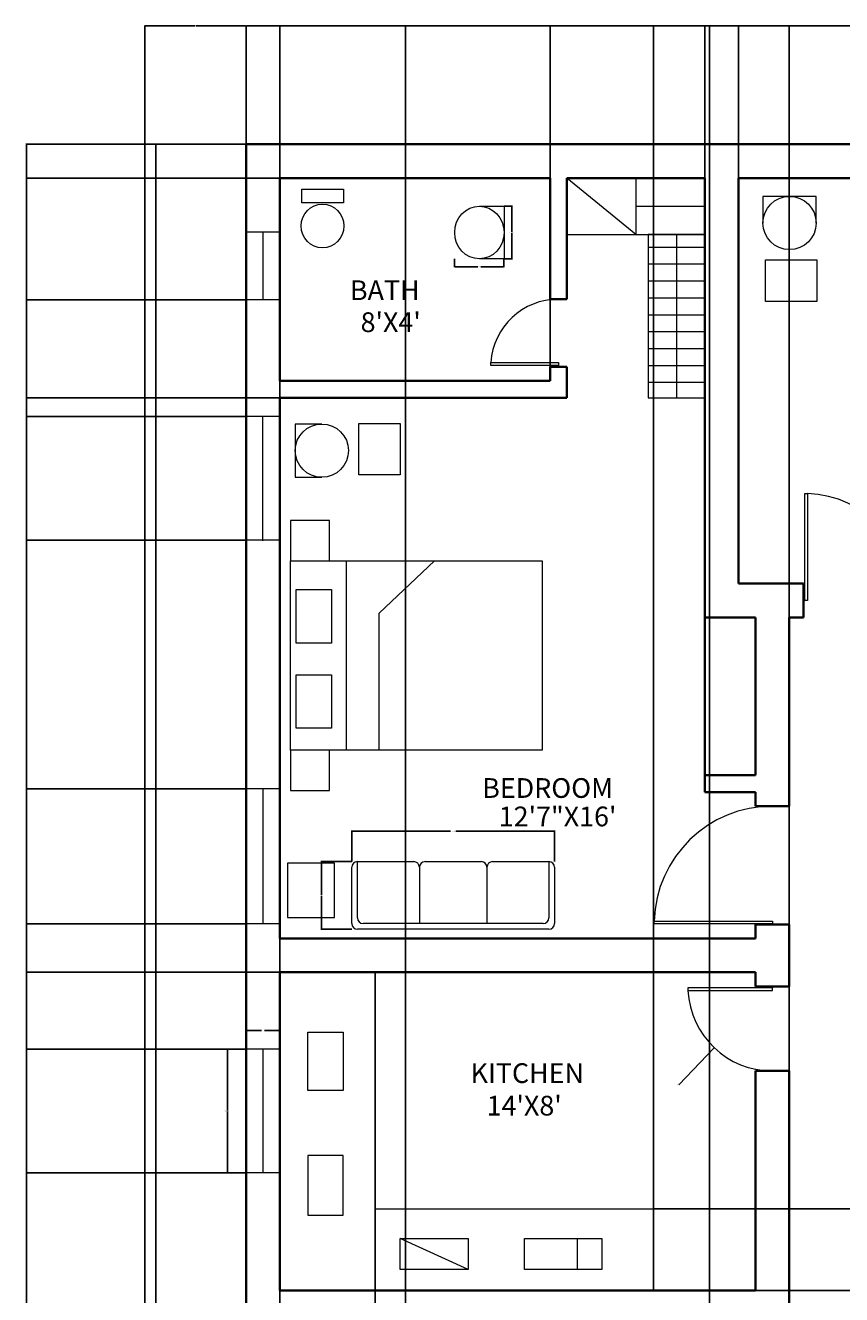
# Model space of a CAD drawing. Units: inches. Extents: x 2863 to 3499, y 1212 to 2136.
# Tile 5 of 7: x 2863 to 3153, y 1686 to 2136. Entities that reach past the tile are written whole.
import ezdxf

# ---------------------------------------------------------------- set-up
doc = ezdxf.new("R2010")
doc.units = ezdxf.units.IN
for name, color, linetype, lineweight in [('A-ANNO-DIMS', 2, 'Continuous', 18), ('A-AREA-IDEN', 7, 'Continuous', 18), ('A-DOOR', 221, 'Continuous', 18), ('A-FLOR-CASE', 254, 'Continuous', 18), ('A-FLOR-FIXT', 254, 'Continuous', 18), ('A-FURN', 131, 'Continuous', 18), ('A-GLAZ', 191, 'Continuous', 18), ('A-WALL', 51, 'Continuous', 35), ('C-PROP', 51, 'Continuous', 25)]:
    doc.layers.add(name, color=color, linetype=linetype, lineweight=lineweight)
doc.styles.get("Standard").update_dxf_attribs({"font": 'arial.ttf'})
doc.dimstyles.get("Standard").update_dxf_attribs({"dimtxt": 0.18, "dimasz": 0.18, "dimexe": 0.18, "dimexo": 0.0625, "dimgap": 0.09, "dimtad": 0, "dimtih": 1, "dimtoh": 1, "dimdec": 4, "dimzin": 0, "dimdsep": 46, "dimtxsty": 'Standard', "dimcen": 0.09, "dimadec": 0, "dimazin": 0, "dimtfac": 1, "dimtdec": 4, "dimtofl": 0, "dimtmove": 0, "dimatfit": 3, "dimfxl": 1, "dimtolj": 1, "dimtzin": 0, "dimarcsym": 0})

# ---------------------------------------------------------------- blocks, each defined once
blk = doc.blocks.new('BED-DOUBLE-WITH-NIGHTSTANDS')
for p, q in [((19.89, 14.28), (19.89, 81.52)), ((31.47, 62.91), (51.09, 81.52)), ((31.47, 14.28), (31.47, 62.91))]:
    blk.add_line(p, q)
for points in [[(0, 81.52), (13.89, 81.52), (13.89, 95.8), (0, 95.8)], [(0, 81.52), (89.37, 81.52), (89.37, 14.28), (0, 14.28)], [(2, 71.31), (14.52, 71.31), (14.52, 52.28), (2, 52.28)], [(2, 41.11), (14.52, 41.11), (14.52, 22.08), (2, 22.08)], [(0, 0), (13.89, 0), (13.89, 14.28), (0, 14.28)]]:
    blk.add_lwpolyline(points, close=True)
blk = doc.blocks.new('WC-CLOSE-COUPLED')
blk.add_lwpolyline([(0.19, 20.82), (15, 20.82), (15, 15.96), (0.19, 15.96)], close=True)
blk.add_ellipse((7.6, 7.79), major_axis=(0, 7.78), ratio=0.975839)
blk = doc.blocks.new('CHAIR-ROUND-BACK')
for p, q in [((18.9, 18.9), (0, 18.9)), ((0, 18.9), (0, 9.45)), ((18.9, 9.45), (18.9, 18.9))]:
    blk.add_line(p, q)
blk.add_circle((9.45, 9.45), 9.45)
blk = doc.blocks.new('TABLE-SIDE-RECT')
blk.add_lwpolyline([(18.23, 14.69), (18.23, 0), (0, 0), (0, 14.69)], close=True)
blk = doc.blocks.new('SOFA-THREE-SEAT')
for p, q in [((2, 24), (22, 24)), ((2, 4), (2, 24)), ((26, 24), (46, 24)), ((50, 24), (70, 24)), ((70, 24), (70, 4)), ((0, 2), (0, 22)), ((24, 22), (24, 2)), ((24, 22), (24, 22)), ((48, 22), (48, 2)), ((48, 22), (48, 22)), ((72, 22), (72, 2)), ((70, 0), (2, 0)), ((68, 2), (4, 2))]:
    blk.add_line(p, q)
for centre, start, end in [((2, 22), 90, 180), ((22, 22), 0, 90), ((26, 22), 90, 180), ((46, 22), 0, 90), ((50, 22), 90, 180), ((70, 22), 0, 90), ((2, 2), 180, 270), ((4, 4), 180, 270), ((68, 4), 270, 0), ((70, 2), 270, 0)]:
    blk.add_arc(centre, 2, start, end)
blk = doc.blocks.new('BASIN-WALL')
for p, q in [((8.77, 18.68), (17.53, 18.68)), ((17.53, 18.68), (17.53, 0)), ((17.53, 0), (8.77, 0))]:
    blk.add_line(p, q)
blk.add_ellipse((8.77, 9.34), major_axis=(0, 9.34), ratio=0.938307)
blk = doc.blocks.new('DOOR-SWING-24IN')
for p, q in [((0, 0.5), (0, 1.5)), ((0, 1.5), (24, 1.5)), ((24, 0.5), (0, 0.5)), ((24, 1.5), (24, 0.5)), ((24, 0), (24, 0.5))]:
    blk.add_line(p, q)
blk.add_arc((23.95, 0), 24, 89.888, 176.4168)
blk = doc.blocks.new('WINDOW-24IN')
for p, q in [((12, 24), (0, 24)), ((6, 24), (6, 0)), ((12, 0), (0, 0))]:
    blk.add_line(p, q)
blk = doc.blocks.new('WINDOW-44IN')
for p, q in [((12, 44), (0, 44)), ((6, 44), (6, 0)), ((12, 0), (0, 0))]:
    blk.add_line(p, q)
blk = doc.blocks.new('WINDOW-48IN')
for p, q in [((12, 48), (0, 48)), ((6, 48), (6, 0)), ((12, 0), (0, 0))]:
    blk.add_line(p, q)
blk = doc.blocks.new('*D29')
at = {"layer": 'A-ANNO-DIMS', "color": 0, "lineweight": -2, "transparency": 16777216}
for p, q in [((3032.63, 2072.16), (3035.55, 2072.16)), ((3035.37, 2071.98), (3035.37, 2063)), ((3035.37, 2053.66), (3035.37, 2062.64)), ((3032.63, 2053.48), (3035.55, 2053.48))]:
    blk.add_line(p, q, dxfattribs=at)
at = {"layer": 'A-ANNO-DIMS', "color": 0, "transparency": 16777216}
for points in [[(3035.34, 2071.98), (3035.4, 2071.98), (3035.37, 2072.16)], [(3035.34, 2053.66), (3035.4, 2053.66), (3035.37, 2053.48)]]:
    blk.add_solid(points, dxfattribs=at)
at = {"layer": 'Defpoints', "color": 0, "transparency": 16777216}
for p in [(3032.56, 2072.16), (3035.37, 2072.16), (3032.56, 2053.48)]:
    blk.add_point(p, dxfattribs=at)
at = {"layer": 'A-ANNO-DIMS', "color": 0, "transparency": 16777216, "insert": (3035.37, 2062.82), "char_height": 0.18, "attachment_point": 5}
blk.add_mtext('\\A1;BASIN 19 TYP.', dxfattribs=at)
blk = doc.blocks.new('*D30')
at = {"layer": 'A-ANNO-DIMS', "color": 0, "lineweight": -2, "transparency": 16777216}
for p, q in [((3015.03, 2053.42), (3015.03, 2050.5)), ((3015.21, 2050.68), (3023.28, 2050.68)), ((3032.38, 2050.68), (3024.32, 2050.68)), ((3032.56, 2053.42), (3032.56, 2050.5))]:
    blk.add_line(p, q, dxfattribs=at)
at = {"layer": 'A-ANNO-DIMS', "color": 0, "transparency": 16777216}
for points in [[(3015.21, 2050.71), (3015.21, 2050.65), (3015.03, 2050.68)], [(3032.38, 2050.71), (3032.38, 2050.65), (3032.56, 2050.68)]]:
    blk.add_solid(points, dxfattribs=at)
at = {"layer": 'Defpoints', "color": 0, "transparency": 16777216}
for p in [(3015.03, 2053.48), (3032.56, 2053.48), (3032.56, 2050.68)]:
    blk.add_point(p, dxfattribs=at)
at = {"layer": 'A-ANNO-DIMS', "color": 0, "transparency": 16777216, "insert": (3023.8, 2050.68), "char_height": 0.18, "attachment_point": 5}
blk.add_mtext('\\A1;18 TYP.', dxfattribs=at)
blk = doc.blocks.new('*D41')
at = {"layer": 'A-ANNO-DIMS', "color": 0, "lineweight": -2, "transparency": 16777216}
for p, q in [((2978.51, 1839.54), (2978.51, 1850.46)), ((2978.69, 1850.28), (3013.61, 1850.28)), ((3050.33, 1850.28), (3015.42, 1850.28)), ((3050.51, 1839.54), (3050.51, 1850.46))]:
    blk.add_line(p, q, dxfattribs=at)
at = {"layer": 'A-ANNO-DIMS', "color": 0, "transparency": 16777216}
for points in [[(2978.69, 1850.31), (2978.69, 1850.25), (2978.51, 1850.28)], [(3050.33, 1850.31), (3050.33, 1850.25), (3050.51, 1850.28)]]:
    blk.add_solid(points, dxfattribs=at)
at = {"layer": 'Defpoints', "color": 0, "transparency": 16777216}
for p in [(3050.51, 1850.28), (2978.51, 1839.48), (3050.51, 1839.48)]:
    blk.add_point(p, dxfattribs=at)
at = {"layer": 'A-ANNO-DIMS', "color": 0, "transparency": 16777216, "insert": (3014.51, 1850.28), "char_height": 0.18, "attachment_point": 5}
blk.add_mtext('\\A1;SOFA 72 TYP.', dxfattribs=at)
blk = doc.blocks.new('*D42')
at = {"layer": 'A-ANNO-DIMS', "color": 0, "lineweight": -2, "transparency": 16777216}
for p, q in [((2978.45, 1839.48), (2967.53, 1839.48)), ((2967.71, 1839.3), (2967.71, 1827.66)), ((2967.71, 1815.66), (2967.71, 1827.3)), ((2978.45, 1815.48), (2967.53, 1815.48))]:
    blk.add_line(p, q, dxfattribs=at)
at = {"layer": 'A-ANNO-DIMS', "color": 0, "transparency": 16777216}
for points in [[(2967.68, 1839.3), (2967.74, 1839.3), (2967.71, 1839.48)], [(2967.68, 1815.66), (2967.74, 1815.66), (2967.71, 1815.48)]]:
    blk.add_solid(points, dxfattribs=at)
at = {"layer": 'Defpoints', "color": 0, "transparency": 16777216}
for p in [(2967.71, 1839.48), (2978.51, 1839.48), (2978.51, 1815.48)]:
    blk.add_point(p, dxfattribs=at)
at = {"layer": 'A-ANNO-DIMS', "color": 0, "transparency": 16777216, "insert": (2967.71, 1827.48), "char_height": 0.18, "attachment_point": 5}
blk.add_mtext('\\A1;24 TYP.', dxfattribs=at)
blk = doc.blocks.new('*D45')
at = {"layer": 'A-ANNO-DIMS', "color": 0, "lineweight": -2, "transparency": 16777216}
for p, q in [((2940.85, 1772.91), (2934.14, 1772.91)), ((2934.32, 1772.73), (2934.32, 1751.1)), ((2934.32, 1729.09), (2934.32, 1750.73)), ((2940.85, 1728.91), (2934.14, 1728.91))]:
    blk.add_line(p, q, dxfattribs=at)
at = {"layer": 'A-ANNO-DIMS', "color": 0, "transparency": 16777216}
for points in [[(2934.29, 1772.73), (2934.35, 1772.73), (2934.32, 1772.91)], [(2934.29, 1729.09), (2934.35, 1729.09), (2934.32, 1728.91)]]:
    blk.add_solid(points, dxfattribs=at)
at = {"layer": 'Defpoints', "color": 0, "transparency": 16777216}
for p in [(2934.32, 1772.91), (2940.92, 1772.91), (2940.92, 1728.91)]:
    blk.add_point(p, dxfattribs=at)
at = {"layer": 'A-ANNO-DIMS', "color": 0, "transparency": 16777216, "insert": (2934.32, 1750.91), "char_height": 0.18, "attachment_point": 5}
blk.add_mtext('\\A1;WINDOW 44 TYP.', dxfattribs=at)
blk = doc.blocks.new('*D46')
at = {"layer": 'A-ANNO-DIMS', "color": 0, "lineweight": -2, "transparency": 16777216}
for p, q in [((2940.92, 1772.98), (2940.92, 1779.69)), ((2941.1, 1779.51), (2946.4, 1779.51)), ((2952.74, 1779.51), (2947.44, 1779.51)), ((2952.92, 1772.98), (2952.92, 1779.69))]:
    blk.add_line(p, q, dxfattribs=at)
at = {"layer": 'A-ANNO-DIMS', "color": 0, "transparency": 16777216}
for points in [[(2941.1, 1779.54), (2941.1, 1779.48), (2940.92, 1779.51)], [(2952.74, 1779.54), (2952.74, 1779.48), (2952.92, 1779.51)]]:
    blk.add_solid(points, dxfattribs=at)
at = {"layer": 'Defpoints', "color": 0, "transparency": 16777216}
for p in [(2952.92, 1779.51), (2940.92, 1772.91), (2952.92, 1772.91)]:
    blk.add_point(p, dxfattribs=at)
at = {"layer": 'A-ANNO-DIMS', "color": 0, "transparency": 16777216, "insert": (2946.92, 1779.51), "char_height": 0.18, "attachment_point": 5}
blk.add_mtext('\\A1;12 TYP.', dxfattribs=at)
blk = doc.blocks.new('*D50')
at = {"layer": 'A-ANNO-DIMS', "color": 0, "lineweight": -2, "transparency": 16777216}
for p, q in [((2904.85, 2094.17), (2862.72, 2094.17)), ((2862.9, 2093.99), (2862.9, 1674.35)), ((2862.9, 1254.35), (2862.9, 1673.98)), ((2904.85, 1254.17), (2862.72, 1254.17))]:
    blk.add_line(p, q, dxfattribs=at)
at = {"layer": 'A-ANNO-DIMS', "color": 0, "transparency": 16777216}
for points in [[(2862.87, 2093.99), (2862.93, 2093.99), (2862.9, 2094.17)], [(2862.87, 1254.35), (2862.93, 1254.35), (2862.9, 1254.17)]]:
    blk.add_solid(points, dxfattribs=at)
at = {"layer": 'Defpoints', "color": 0, "transparency": 16777216}
for p in [(2862.9, 2094.17), (2904.92, 2094.17), (2904.92, 1254.17)]:
    blk.add_point(p, dxfattribs=at)
at = {"layer": 'A-ANNO-DIMS', "color": 0, "transparency": 16777216, "insert": (2862.9, 1674.17), "char_height": 0.18, "attachment_point": 5}
blk.add_mtext('\\A1;840', dxfattribs=at)
blk = doc.blocks.new('*D51')
at = {"layer": 'A-ANNO-DIMS', "color": 0, "lineweight": -2, "transparency": 16777216}
for p, q in [((2904.92, 2094.23), (2904.92, 2136.37)), ((2905.1, 2136.19), (2922.7, 2136.19)), ((2940.74, 2136.19), (2923.14, 2136.19)), ((2940.92, 2094.23), (2940.92, 2136.37))]:
    blk.add_line(p, q, dxfattribs=at)
at = {"layer": 'A-ANNO-DIMS', "color": 0, "transparency": 16777216}
for points in [[(2905.1, 2136.22), (2905.1, 2136.16), (2904.92, 2136.19)], [(2940.74, 2136.22), (2940.74, 2136.16), (2940.92, 2136.19)]]:
    blk.add_solid(points, dxfattribs=at)
at = {"layer": 'Defpoints', "color": 0, "transparency": 16777216}
for p in [(2940.92, 2136.19), (2904.92, 2094.17), (2940.92, 2094.17)]:
    blk.add_point(p, dxfattribs=at)
at = {"layer": 'A-ANNO-DIMS', "color": 0, "transparency": 16777216, "insert": (2922.92, 2136.19), "char_height": 0.18, "attachment_point": 5}
blk.add_mtext('\\A1;36', dxfattribs=at)
blk = doc.blocks.new('*D52')
at = {"layer": 'A-ANNO-DIMS', "color": 0, "lineweight": -2, "transparency": 16777216}
for p, q in [((2940.92, 2094.23), (2940.92, 2136.37)), ((2941.1, 2136.19), (3180.62, 2136.19)), ((3420.74, 2136.19), (3181.21, 2136.19)), ((3420.92, 2094.23), (3420.92, 2136.37))]:
    blk.add_line(p, q, dxfattribs=at)
at = {"layer": 'A-ANNO-DIMS', "color": 0, "transparency": 16777216}
for points in [[(2941.1, 2136.22), (2941.1, 2136.16), (2940.92, 2136.19)], [(3420.74, 2136.22), (3420.74, 2136.16), (3420.92, 2136.19)]]:
    blk.add_solid(points, dxfattribs=at)
at = {"layer": 'Defpoints', "color": 0, "transparency": 16777216}
for p in [(3420.92, 2136.19), (2940.92, 2094.17), (3420.92, 2094.17)]:
    blk.add_point(p, dxfattribs=at)
at = {"layer": 'A-ANNO-DIMS', "color": 0, "transparency": 16777216, "insert": (3180.92, 2136.19), "char_height": 0.18, "attachment_point": 5}
blk.add_mtext('\\A1;480', dxfattribs=at)
blk = doc.blocks.new('*D54')
at = {"layer": 'A-ANNO-DIMS', "color": 0, "lineweight": -2, "transparency": 16777216}
for p, q in [((2952.92, 2082.23), (2952.92, 2136.37)), ((2953.1, 2136.19), (3028.15, 2136.19)), ((3103.74, 2136.19), (3028.68, 2136.19)), ((3103.92, 2082.23), (3103.92, 2136.37))]:
    blk.add_line(p, q, dxfattribs=at)
at = {"layer": 'A-ANNO-DIMS', "color": 0, "transparency": 16777216}
for points in [[(2953.1, 2136.22), (2953.1, 2136.16), (2952.92, 2136.19)], [(3103.74, 2136.22), (3103.74, 2136.16), (3103.92, 2136.19)]]:
    blk.add_solid(points, dxfattribs=at)
at = {"layer": 'Defpoints', "color": 0, "transparency": 16777216}
for p in [(3103.92, 2136.19), (2952.92, 2082.17), (3103.92, 2082.17)]:
    blk.add_point(p, dxfattribs=at)
at = {"layer": 'A-ANNO-DIMS', "color": 0, "transparency": 16777216, "insert": (3028.42, 2136.19), "char_height": 0.18, "attachment_point": 5}
blk.add_mtext('\\A1;151', dxfattribs=at)
blk = doc.blocks.new('*D55')
at = {"layer": 'A-ANNO-DIMS', "color": 0, "lineweight": -2, "transparency": 16777216}
for p, q in [((3115.92, 2082.23), (3115.92, 2136.37)), ((3116.1, 2136.19), (3211.64, 2136.19)), ((3307.74, 2136.19), (3212.2, 2136.19)), ((3307.92, 2082.23), (3307.92, 2136.37))]:
    blk.add_line(p, q, dxfattribs=at)
at = {"layer": 'A-ANNO-DIMS', "color": 0, "transparency": 16777216}
for points in [[(3116.1, 2136.22), (3116.1, 2136.16), (3115.92, 2136.19)], [(3307.74, 2136.22), (3307.74, 2136.16), (3307.92, 2136.19)]]:
    blk.add_solid(points, dxfattribs=at)
at = {"layer": 'Defpoints', "color": 0, "transparency": 16777216}
for p in [(3307.92, 2136.19), (3115.92, 2082.17), (3307.92, 2082.17)]:
    blk.add_point(p, dxfattribs=at)
at = {"layer": 'A-ANNO-DIMS', "color": 0, "transparency": 16777216, "insert": (3211.92, 2136.19), "char_height": 0.18, "attachment_point": 5}
blk.add_mtext('\\A1;192', dxfattribs=at)
blk = doc.blocks.new('*D66')
at = {"layer": 'A-ANNO-DIMS', "color": 0, "lineweight": -2, "transparency": 16777216}
for p, q in [((2952.85, 1800.17), (2862.72, 1800.17)), ((2862.9, 1799.99), (2862.9, 1737.85)), ((2862.9, 1675.35), (2862.9, 1737.48)), ((2952.85, 1675.17), (2862.72, 1675.17))]:
    blk.add_line(p, q, dxfattribs=at)
at = {"layer": 'A-ANNO-DIMS', "color": 0, "transparency": 16777216}
for points in [[(2862.87, 1799.99), (2862.93, 1799.99), (2862.9, 1800.17)], [(2862.87, 1675.35), (2862.93, 1675.35), (2862.9, 1675.17)]]:
    blk.add_solid(points, dxfattribs=at)
at = {"layer": 'Defpoints', "color": 0, "transparency": 16777216}
for p in [(2862.9, 1800.17), (2952.92, 1800.17), (2952.92, 1675.17)]:
    blk.add_point(p, dxfattribs=at)
at = {"layer": 'A-ANNO-DIMS', "color": 0, "transparency": 16777216, "insert": (2862.9, 1737.67), "char_height": 0.18, "attachment_point": 5}
blk.add_mtext('\\A1;125', dxfattribs=at)
blk = doc.blocks.new('*D67')
at = {"layer": 'A-ANNO-DIMS', "color": 0, "lineweight": -2, "transparency": 16777216}
for p, q in [((2952.85, 2004.17), (2862.72, 2004.17)), ((2862.9, 2003.99), (2862.9, 1902.35)), ((2862.9, 1800.35), (2862.9, 1901.98)), ((2952.85, 1800.17), (2862.72, 1800.17))]:
    blk.add_line(p, q, dxfattribs=at)
at = {"layer": 'A-ANNO-DIMS', "color": 0, "transparency": 16777216}
for points in [[(2862.87, 2003.99), (2862.93, 2003.99), (2862.9, 2004.17)], [(2862.87, 1800.35), (2862.93, 1800.35), (2862.9, 1800.17)]]:
    blk.add_solid(points, dxfattribs=at)
at = {"layer": 'Defpoints', "color": 0, "transparency": 16777216}
for p in [(2862.9, 2004.17), (2952.92, 2004.17), (2952.92, 1800.17)]:
    blk.add_point(p, dxfattribs=at)
at = {"layer": 'A-ANNO-DIMS', "color": 0, "transparency": 16777216, "insert": (2862.9, 1902.17), "char_height": 0.18, "attachment_point": 5}
blk.add_mtext('\\A1;204', dxfattribs=at)
blk = doc.blocks.new('*D68')
at = {"layer": 'A-ANNO-DIMS', "color": 0, "lineweight": -2, "transparency": 16777216}
for p, q in [((2952.85, 2082.17), (2862.72, 2082.17)), ((2862.9, 2081.99), (2862.9, 2043.35)), ((2862.9, 2004.35), (2862.9, 2042.98)), ((2952.85, 2004.17), (2862.72, 2004.17))]:
    blk.add_line(p, q, dxfattribs=at)
at = {"layer": 'A-ANNO-DIMS', "color": 0, "transparency": 16777216}
for points in [[(2862.87, 2081.99), (2862.93, 2081.99), (2862.9, 2082.17)], [(2862.87, 2004.35), (2862.93, 2004.35), (2862.9, 2004.17)]]:
    blk.add_solid(points, dxfattribs=at)
at = {"layer": 'Defpoints', "color": 0, "transparency": 16777216}
for p in [(2862.9, 2082.17), (2952.92, 2082.17), (2952.92, 2004.17)]:
    blk.add_point(p, dxfattribs=at)
at = {"layer": 'A-ANNO-DIMS', "color": 0, "transparency": 16777216, "insert": (2862.9, 2043.17), "char_height": 0.18, "attachment_point": 5}
blk.add_mtext('\\A1;78', dxfattribs=at)
blk = doc.blocks.new('*D72')
at = {"layer": 'A-ANNO-DIMS', "color": 0, "lineweight": -2, "transparency": 16777216}
for p, q in [((3133.92, 1549.23), (3133.92, 2136.37)), ((3134.1, 2136.19), (3169.22, 2136.19)), ((3204.74, 2136.19), (3169.62, 2136.19)), ((3204.92, 1561.23), (3204.92, 2136.37))]:
    blk.add_line(p, q, dxfattribs=at)
at = {"layer": 'A-ANNO-DIMS', "color": 0, "transparency": 16777216}
for points in [[(3134.1, 2136.22), (3134.1, 2136.16), (3133.92, 2136.19)], [(3204.74, 2136.22), (3204.74, 2136.16), (3204.92, 2136.19)]]:
    blk.add_solid(points, dxfattribs=at)
at = {"layer": 'Defpoints', "color": 0, "transparency": 16777216}
for p in [(3204.92, 2136.19), (3204.92, 1561.17), (3133.92, 1549.17)]:
    blk.add_point(p, dxfattribs=at)
at = {"layer": 'A-ANNO-DIMS', "color": 0, "transparency": 16777216, "insert": (3169.42, 2136.19), "char_height": 0.18, "attachment_point": 5}
blk.add_mtext('\\A1;71', dxfattribs=at)
blk = doc.blocks.new('*D75')
at = {"layer": 'A-ANNO-DIMS', "color": 0, "lineweight": -2, "transparency": 16777216}
for p, q in [((2952.92, 2010.23), (2952.92, 2136.37)), ((2953.1, 2136.19), (3000.7, 2136.19)), ((3048.74, 2136.19), (3001.14, 2136.19)), ((3048.92, 2010.23), (3048.92, 2136.37))]:
    blk.add_line(p, q, dxfattribs=at)
at = {"layer": 'A-ANNO-DIMS', "color": 0, "transparency": 16777216}
for points in [[(2953.1, 2136.22), (2953.1, 2136.16), (2952.92, 2136.19)], [(3048.74, 2136.22), (3048.74, 2136.16), (3048.92, 2136.19)]]:
    blk.add_solid(points, dxfattribs=at)
at = {"layer": 'Defpoints', "color": 0, "transparency": 16777216}
for p in [(3048.92, 2136.19), (2952.92, 2010.17), (3048.92, 2010.17)]:
    blk.add_point(p, dxfattribs=at)
at = {"layer": 'A-ANNO-DIMS', "color": 0, "transparency": 16777216, "insert": (3000.92, 2136.19), "char_height": 0.18, "attachment_point": 5}
blk.add_mtext('\\A1;96', dxfattribs=at)
blk = doc.blocks.new('*D77')
at = {"layer": 'A-ANNO-DIMS', "color": 0, "lineweight": -2, "transparency": 16777216}
for p, q in [((2997.55, 1549.23), (2997.55, 2136.37)), ((2997.73, 2136.19), (3051.27, 2136.19)), ((3105.37, 2136.19), (3051.83, 2136.19)), ((3105.55, 1549.23), (3105.55, 2136.37))]:
    blk.add_line(p, q, dxfattribs=at)
at = {"layer": 'A-ANNO-DIMS', "color": 0, "transparency": 16777216}
for points in [[(2997.73, 2136.22), (2997.73, 2136.16), (2997.55, 2136.19)], [(3105.37, 2136.22), (3105.37, 2136.16), (3105.55, 2136.19)]]:
    blk.add_solid(points, dxfattribs=at)
at = {"layer": 'Defpoints', "color": 0, "transparency": 16777216}
for p in [(3105.55, 2136.19), (2997.55, 1549.17), (3105.55, 1549.17)]:
    blk.add_point(p, dxfattribs=at)
at = {"layer": 'A-ANNO-DIMS', "color": 0, "transparency": 16777216, "insert": (3051.55, 2136.19), "char_height": 0.18, "attachment_point": 5}
blk.add_mtext('\\A1;108', dxfattribs=at)
blk = doc.blocks.new('*D78')
at = {"layer": 'A-ANNO-DIMS', "color": 0, "lineweight": -2, "transparency": 16777216}
for p, q in [((2952.92, 1687.23), (2952.92, 2136.37)), ((2953.1, 2136.19), (3018.83, 2136.19)), ((3085.47, 2136.19), (3019.74, 2136.19)), ((3085.65, 1687.23), (3085.65, 2136.37))]:
    blk.add_line(p, q, dxfattribs=at)
at = {"layer": 'A-ANNO-DIMS', "color": 0, "transparency": 16777216}
for points in [[(2953.1, 2136.22), (2953.1, 2136.16), (2952.92, 2136.19)], [(3085.47, 2136.22), (3085.47, 2136.16), (3085.65, 2136.19)]]:
    blk.add_solid(points, dxfattribs=at)
at = {"layer": 'Defpoints', "color": 0, "transparency": 16777216}
for p in [(3085.65, 2136.19), (2952.92, 1687.17), (3085.65, 1687.17)]:
    blk.add_point(p, dxfattribs=at)
at = {"layer": 'A-ANNO-DIMS', "color": 0, "transparency": 16777216, "insert": (3019.29, 2136.19), "char_height": 0.18, "attachment_point": 5}
blk.add_mtext('\\A1;132.74', dxfattribs=at)
blk = doc.blocks.new('*D86')
at = {"layer": 'A-ANNO-DIMS', "color": 0, "lineweight": -2, "transparency": 16777216}
for p, q in [((2940.85, 1728.91), (2862.72, 1728.91)), ((2862.9, 1728.73), (2862.9, 1690.09)), ((2862.9, 1651.09), (2862.9, 1689.73)), ((2940.85, 1650.91), (2862.72, 1650.91))]:
    blk.add_line(p, q, dxfattribs=at)
at = {"layer": 'A-ANNO-DIMS', "color": 0, "transparency": 16777216}
for points in [[(2862.87, 1728.73), (2862.93, 1728.73), (2862.9, 1728.91)], [(2862.87, 1651.09), (2862.93, 1651.09), (2862.9, 1650.91)]]:
    blk.add_solid(points, dxfattribs=at)
at = {"layer": 'Defpoints', "color": 0, "transparency": 16777216}
for p in [(2862.9, 1728.91), (2940.92, 1728.91), (2940.92, 1650.91)]:
    blk.add_point(p, dxfattribs=at)
at = {"layer": 'A-ANNO-DIMS', "color": 0, "transparency": 16777216, "insert": (2862.9, 1689.91), "char_height": 0.18, "attachment_point": 5}
blk.add_mtext('\\A1;78', dxfattribs=at)
blk = doc.blocks.new('*D87')
at = {"layer": 'A-ANNO-DIMS', "color": 0, "lineweight": -2, "transparency": 16777216}
for p, q in [((2940.85, 1817.32), (2862.72, 1817.32)), ((2862.9, 1817.14), (2862.9, 1795.3)), ((2862.9, 1773.09), (2862.9, 1794.94)), ((2940.85, 1772.91), (2862.72, 1772.91))]:
    blk.add_line(p, q, dxfattribs=at)
at = {"layer": 'A-ANNO-DIMS', "color": 0, "transparency": 16777216}
for points in [[(2862.87, 1817.14), (2862.93, 1817.14), (2862.9, 1817.32)], [(2862.87, 1773.09), (2862.93, 1773.09), (2862.9, 1772.91)]]:
    blk.add_solid(points, dxfattribs=at)
at = {"layer": 'Defpoints', "color": 0, "transparency": 16777216}
for p in [(2862.9, 1817.32), (2940.92, 1817.32), (2940.92, 1772.91)]:
    blk.add_point(p, dxfattribs=at)
at = {"layer": 'A-ANNO-DIMS', "color": 0, "transparency": 16777216, "insert": (2862.9, 1795.12), "char_height": 0.18, "attachment_point": 5}
blk.add_mtext('\\A1;44.41', dxfattribs=at)
blk = doc.blocks.new('*D88')
at = {"layer": 'A-ANNO-DIMS', "color": 0, "lineweight": -2, "transparency": 16777216}
for p, q in [((2940.85, 1953.55), (2862.72, 1953.55)), ((2862.9, 1953.37), (2862.9, 1909.62)), ((2862.9, 1865.5), (2862.9, 1909.26)), ((2940.85, 1865.32), (2862.72, 1865.32))]:
    blk.add_line(p, q, dxfattribs=at)
at = {"layer": 'A-ANNO-DIMS', "color": 0, "transparency": 16777216}
for points in [[(2862.87, 1953.37), (2862.93, 1953.37), (2862.9, 1953.55)], [(2862.87, 1865.5), (2862.93, 1865.5), (2862.9, 1865.32)]]:
    blk.add_solid(points, dxfattribs=at)
at = {"layer": 'Defpoints', "color": 0, "transparency": 16777216}
for p in [(2862.9, 1953.55), (2940.92, 1953.55), (2940.92, 1865.32)]:
    blk.add_point(p, dxfattribs=at)
at = {"layer": 'A-ANNO-DIMS', "color": 0, "transparency": 16777216, "insert": (2862.9, 1909.44), "char_height": 0.18, "attachment_point": 5}
blk.add_mtext('\\A1;88.23', dxfattribs=at)
blk = doc.blocks.new('*D89')
at = {"layer": 'A-ANNO-DIMS', "color": 0, "lineweight": -2, "transparency": 16777216}
for p, q in [((2940.85, 2038.97), (2862.72, 2038.97)), ((2862.9, 2038.79), (2862.9, 2018.44)), ((2862.9, 1997.73), (2862.9, 2018.08)), ((2940.85, 1997.55), (2862.72, 1997.55))]:
    blk.add_line(p, q, dxfattribs=at)
at = {"layer": 'A-ANNO-DIMS', "color": 0, "transparency": 16777216}
for points in [[(2862.87, 2038.79), (2862.93, 2038.79), (2862.9, 2038.97)], [(2862.87, 1997.73), (2862.93, 1997.73), (2862.9, 1997.55)]]:
    blk.add_solid(points, dxfattribs=at)
at = {"layer": 'Defpoints', "color": 0, "transparency": 16777216}
for p in [(2862.9, 2038.97), (2940.92, 2038.97), (2940.92, 1997.55)]:
    blk.add_point(p, dxfattribs=at)
at = {"layer": 'A-ANNO-DIMS', "color": 0, "transparency": 16777216, "insert": (2862.9, 2018.26), "char_height": 0.18, "attachment_point": 5}
blk.add_mtext('\\A1;41.414', dxfattribs=at)
blk = doc.blocks.new('*D111')
at = {"layer": 'A-ANNO-DIMS', "color": 0, "lineweight": -2, "transparency": 16777216}
for p, q in [((2952.92, 1549.23), (2952.92, 2136.37)), ((2953.1, 2136.19), (2974.83, 2136.19)), ((2997.37, 2136.19), (2975.63, 2136.19)), ((2997.55, 1549.23), (2997.55, 2136.37))]:
    blk.add_line(p, q, dxfattribs=at)
at = {"layer": 'A-ANNO-DIMS', "color": 0, "transparency": 16777216}
for points in [[(2953.1, 2136.22), (2953.1, 2136.16), (2952.92, 2136.19)], [(2997.37, 2136.22), (2997.37, 2136.16), (2997.55, 2136.19)]]:
    blk.add_solid(points, dxfattribs=at)
at = {"layer": 'Defpoints', "color": 0, "transparency": 16777216}
for p in [(2997.55, 2136.19), (2952.92, 1549.17), (2997.55, 1549.17)]:
    blk.add_point(p, dxfattribs=at)
at = {"layer": 'A-ANNO-DIMS', "color": 0, "transparency": 16777216, "insert": (2975.23, 2136.19), "char_height": 0.18, "attachment_point": 5}
blk.add_mtext('\\A1;44.63', dxfattribs=at)
blk = doc.blocks.new('*D112')
at = {"layer": 'A-ANNO-DIMS', "color": 0, "lineweight": -2, "transparency": 16777216}
for p, q in [((2952.92, 1800.1), (2952.92, 1211.97)), ((2986.74, 1800.1), (2986.74, 1211.97)), ((2953.1, 1212.15), (2969.37, 1212.15)), ((2986.56, 1212.15), (2970.29, 1212.15))]:
    blk.add_line(p, q, dxfattribs=at)
at = {"layer": 'A-ANNO-DIMS', "color": 0, "transparency": 16777216}
for points in [[(2953.1, 1212.18), (2953.1, 1212.12), (2952.92, 1212.15)], [(2986.56, 1212.18), (2986.56, 1212.12), (2986.74, 1212.15)]]:
    blk.add_solid(points, dxfattribs=at)
at = {"layer": 'Defpoints', "color": 0, "transparency": 16777216}
for p in [(2952.92, 1800.17), (2986.74, 1800.17), (2986.74, 1212.15)]:
    blk.add_point(p, dxfattribs=at)
at = {"layer": 'A-ANNO-DIMS', "color": 0, "transparency": 16777216, "insert": (2969.83, 1212.15), "char_height": 0.18, "attachment_point": 5}
blk.add_mtext('\\A1;33.825', dxfattribs=at)
blk = doc.blocks.new('*D113')
at = {"layer": 'A-ANNO-DIMS', "color": 0, "lineweight": -2, "transparency": 16777216}
for p, q in [((3085.72, 1716.17), (3499.12, 1716.17)), ((3498.94, 1715.99), (3498.94, 1701.85)), ((3498.94, 1687.35), (3498.94, 1701.48)), ((3085.72, 1687.17), (3499.12, 1687.17))]:
    blk.add_line(p, q, dxfattribs=at)
at = {"layer": 'A-ANNO-DIMS', "color": 0, "transparency": 16777216}
for points in [[(3498.91, 1715.99), (3498.97, 1715.99), (3498.94, 1716.17)], [(3498.91, 1687.35), (3498.97, 1687.35), (3498.94, 1687.17)]]:
    blk.add_solid(points, dxfattribs=at)
at = {"layer": 'Defpoints', "color": 0, "transparency": 16777216}
for p in [(3085.65, 1716.17), (3498.94, 1716.17), (3085.65, 1687.17)]:
    blk.add_point(p, dxfattribs=at)
at = {"layer": 'A-ANNO-DIMS', "color": 0, "transparency": 16777216, "insert": (3498.94, 1701.67), "char_height": 0.18, "attachment_point": 5}
blk.add_mtext('\\A1;29', dxfattribs=at)
blk = doc.blocks.new('*D114')
at = {"layer": 'A-ANNO-DIMS', "color": 0, "lineweight": -2, "transparency": 16777216}
for p, q in [((3182.77, 1974.31), (3166.45, 1958.64)), ((3182.95, 1974.31), (3182.77, 1974.31)), ((3138.83, 1932.19), (3139.01, 1932.19)), ((3138.92, 1932.1), (3138.92, 1932.28))]:
    blk.add_line(p, q, dxfattribs=at)
at = {"layer": 'A-ANNO-DIMS', "color": 0, "transparency": 16777216}
blk.add_solid([(3166.43, 1958.66), (3166.47, 1958.62), (3166.32, 1958.52)], dxfattribs=at)
at = {"layer": 'Defpoints', "color": 0, "transparency": 16777216}
for p in [(3166.32, 1958.52), (3138.92, 1932.19)]:
    blk.add_point(p, dxfattribs=at)
at = {"layer": 'A-ANNO-DIMS', "color": 0, "transparency": 16777216, "insert": (3183.45, 1974.31), "char_height": 0.18, "attachment_point": 5}
blk.add_mtext('\\A1;2X R38', dxfattribs=at)
blk = doc.blocks.new('*D117')
at = {"layer": 'A-ANNO-DIMS', "color": 0, "lineweight": -2, "transparency": 16777216}
for p, q in [((3127.79, 1795.17), (3127.97, 1795.17)), ((3127.88, 1795.08), (3127.88, 1795.26)), ((3094.82, 1760.36), (3107.09, 1773.28)), ((3094.64, 1760.36), (3094.82, 1760.36))]:
    blk.add_line(p, q, dxfattribs=at)
at = {"layer": 'A-ANNO-DIMS', "color": 0, "transparency": 16777216}
blk.add_solid([(3107.07, 1773.31), (3107.11, 1773.26), (3107.22, 1773.41)], dxfattribs=at)
at = {"layer": 'Defpoints', "color": 0, "transparency": 16777216}
for p in [(3127.88, 1795.17), (3107.22, 1773.41)]:
    blk.add_point(p, dxfattribs=at)
at = {"layer": 'A-ANNO-DIMS', "color": 0, "transparency": 16777216, "insert": (3094.33, 1760.36), "char_height": 0.18, "attachment_point": 5}
blk.add_mtext('\\A1;R30', dxfattribs=at)

msp = doc.modelspace()

# ---------------------------------------------------------------- linework, layer by layer
at = {"layer": 'A-DOOR'}
for p, q in [((3139.4168, 1932.1651), (3139.4168, 1970.1651)), ((3139.4168, 1970.1651), (3140.4168, 1970.1651)), ((3140.4168, 1970.1651), (3140.4168, 1932.1651)), ((3138.9168, 1932.1651), (3139.4168, 1932.1651)), ((3140.4168, 1932.1651), (3138.9168, 1932.1651)), ((3085.9168, 1817.3651), (3085.9168, 1818.3651)), ((3085.9168, 1818.3651), (3127.9168, 1818.3651)), ((3127.9168, 1817.3651), (3085.9168, 1817.3651)), ((3127.9168, 1818.3651), (3127.9168, 1817.3651)), ((3127.9168, 1817.1651), (3127.9168, 1817.3651)), ((3127.9168, 1794.6651), (3097.9168, 1794.6651)), ((3097.9168, 1794.6651), (3097.9168, 1793.6651)), ((3097.9168, 1793.6651), (3127.9168, 1793.6651)), ((3127.9168, 1795.1651), (3127.9168, 1794.6651)), ((3127.9168, 1793.6651), (3127.9168, 1794.6651))]:
    msp.add_line(p, q, dxfattribs=at)
for centre, radius, start, end in [((3138.9168, 1932.1947), 38, 359.955345, 87.737754), ((3127.8996, 1817.1651), 42, 89.976609, 178.36276), ((3127.8792, 1795.1651), 30, 182.865939, 270.071662)]:
    msp.add_arc(centre, radius, start, end, dxfattribs=at)
at = {"layer": 'A-FLOR-CASE'}
for p, q in [((3054.9168, 2082.1651), (3054.9168, 2062.1651)), ((3054.9168, 2082.1651), (3103.9168, 2082.1651)), ((3079.4168, 2062.1651), (3054.9168, 2082.1651)), ((3079.4168, 2082.1651), (3079.4168, 2062.1651)), ((3103.9168, 2082.1651), (3103.9168, 2062.1651)), ((3079.4168, 2072.1651), (3103.9168, 2072.1651)), ((3054.9168, 2062.1651), (3103.9168, 2062.1651)), ((3093.8474, 2062.1651), (3093.8474, 2004.1651)), ((3083.778, 2057.6516), (3103.9168, 2057.6516)), ((3083.778, 2051.6516), (3103.9168, 2051.6516)), ((3083.778, 2045.6516), (3103.9168, 2045.6516)), ((3083.778, 2039.6516), (3103.9168, 2039.6516)), ((3083.778, 2033.6516), (3103.9168, 2033.6516)), ((3083.778, 2027.6516), (3103.9168, 2027.6516)), ((3083.778, 2021.6516), (3103.9168, 2021.6516)), ((3083.778, 2015.6516), (3103.9168, 2015.6516)), ((3083.778, 2009.6516), (3103.9168, 2009.6516)), ((2986.7418, 1800.1651), (2986.7418, 1716.1651)), ((2986.7418, 1716.1651), (3085.6548, 1716.1651)), ((3085.6548, 1716.1651), (3085.6548, 1687.1651))]:
    msp.add_line(p, q, dxfattribs=at)
msp.add_lwpolyline([(3103.9168, 2062.1651), (3083.778, 2062.1651), (3083.778, 2004.1651), (3103.9168, 2004.1651)], close=True, dxfattribs=at)
at = {"layer": 'A-FLOR-FIXT'}
for p, q in [((3019.8674, 1694.5836), (2995.6415, 1705.7049)), ((3058.5472, 1705.7049), (3058.5472, 1694.5836))]:
    msp.add_line(p, q, dxfattribs=at)
for points in [[(2962.8434, 1778.9145), (2975.4564, 1778.9145), (2975.4564, 1758.1651), (2962.8434, 1758.1651)], [(2975.4564, 1735.1383), (2962.8434, 1735.1383), (2962.8434, 1713.9135), (2975.4564, 1713.9135)], [(2995.6415, 1705.7049), (3019.8674, 1705.7049), (3019.8674, 1694.5836), (2995.6415, 1694.5836)], [(3039.8375, 1705.7049), (3067.3372, 1705.7049), (3067.3372, 1694.5836), (3039.8375, 1694.5836)]]:
    msp.add_lwpolyline(points, close=True, dxfattribs=at)
at = {"layer": 'A-FURN'}
msp.add_lwpolyline([(2955.6611, 1819.6484), (2972.3758, 1819.6484), (2972.3758, 1838.9617), (2955.6611, 1838.9617)], close=True, dxfattribs=at)
at = {"layer": 'A-GLAZ'}
for p, q in [((2952.9168, 1997.5533), (2940.9168, 1997.5533)), ((2946.9168, 1953.3818), (2946.9168, 1997.5533)), ((2952.9168, 1953.5533), (2940.9168, 1953.5533))]:
    msp.add_line(p, q, dxfattribs=at)
at = {"layer": 'A-WALL'}
for p, q in [((2952.9168, 2082.1651), (3048.9168, 2082.1651)), ((2952.9168, 2010.1651), (2952.9168, 2082.1651)), ((3048.9168, 2039.1651), (3048.9168, 2082.1651)), ((3054.9168, 2082.1651), (3103.9168, 2082.1651)), ((3054.9168, 2039.1651), (3054.9168, 2082.1651)), ((3103.9168, 1864.1651), (3103.9168, 2082.1651)), ((3115.9168, 2082.1651), (3307.9168, 2082.1651)), ((3115.9168, 1938.1651), (3115.9168, 2082.1651)), ((3054.9168, 2039.1651), (3048.9168, 2039.1651)), ((3048.9168, 2010.1651), (3048.9168, 2015.1651)), ((3054.9168, 2015.1651), (3048.9168, 2015.1651)), ((3054.9168, 2010.1651), (3054.9168, 2015.1651)), ((3054.9168, 2010.1651), (3054.9168, 2015.1651)), ((2952.9168, 2010.1651), (3048.9168, 2010.1651)), ((3054.9168, 2004.1651), (3054.9168, 2010.1651)), ((2952.9168, 2004.1651), (3054.9168, 2004.1651)), ((2952.9168, 1812.1651), (2952.9168, 2004.1651)), ((3115.9168, 1938.1651), (3138.9168, 1938.1651)), ((3138.9168, 1926.1651), (3138.9168, 1938.1651)), ((3103.9168, 1926.1651), (3121.9168, 1926.1651)), ((3103.9168, 1926.1651), (3121.9168, 1926.1651)), ((3121.9168, 1926.1651), (3121.9168, 1870.1651)), ((3133.9168, 1859.1651), (3133.9168, 1926.1651)), ((3133.9168, 1926.1651), (3138.9168, 1926.1651)), ((3103.9168, 1870.1651), (3121.9168, 1870.1651)), ((3121.9168, 1864.1651), (3103.9168, 1864.1651)), ((3121.9168, 1864.1651), (3121.9168, 1859.1651)), ((3121.9168, 1859.1651), (3133.9168, 1859.1651)), ((3133.9168, 1817.1651), (3121.9168, 1817.1651)), ((3121.9168, 1817.1651), (3121.9168, 1812.1651)), ((3133.9168, 1817.1651), (3133.9168, 1800.1651)), ((2952.9168, 1812.1651), (3121.9168, 1812.1651)), ((2952.9168, 1800.1651), (3121.9168, 1800.1651)), ((2952.9168, 1687.1651), (2952.9168, 1800.1651)), ((3121.9168, 1795.1651), (3121.9168, 1800.1651)), ((3133.9168, 1800.1651), (3133.9168, 1795.1651)), ((3133.9168, 1795.1651), (3121.9168, 1795.1651)), ((3121.9168, 1765.1651), (3121.9168, 1687.1651)), ((3133.9168, 1765.1651), (3121.9168, 1765.1651)), ((3133.9168, 1765.1651), (3133.9168, 1687.1651)), ((3121.9168, 1687.1651), (2952.9168, 1687.1651)), ((3133.9168, 1687.1651), (3133.9168, 1675.1651))]:
    msp.add_line(p, q, dxfattribs=at)
msp.add_lwpolyline([(2940.9168, 1453.1651), (2940.9168, 2094.1651), (3420.9168, 2094.1651), (3420.9168, 1374.1651), (3216.9168, 1374.1651)], dxfattribs=at)
at = {"layer": 'C-PROP'}
for p, q in [((2904.9168, 2094.1651), (3456.9168, 2094.1651)), ((2904.9168, 1254.1651), (2904.9168, 2094.1651)), ((2904.9168, 2094.1651), (2940.9168, 2094.1651)), ((2904.9168, 2094.1651), (2908.9168, 2094.1651)), ((2908.9168, 2094.1651), (2908.9168, 1258.1651))]:
    msp.add_line(p, q, dxfattribs=at)

# ---------------------------------------------------------------- block references
at = {"layer": 'A-DOOR'}
msp.add_blockref('DOOR-SWING-24IN', (3027.917, 2015.165), dxfattribs=at)
at = {"layer": 'A-FLOR-FIXT'}
for name, p in [('WC-CLOSE-COUPLED', (2960.492, 2057.371)), ('BASIN-WALL', (3015.033, 2053.479))]:
    msp.add_blockref(name, p, dxfattribs=at)
at = {"layer": 'A-FURN'}
for name, p in [('CHAIR-ROUND-BACK', (3124.55, 2056.751)), ('TABLE-SIDE-RECT', (3125.439, 2038.386)), ('BED-DOUBLE-WITH-NIGHTSTANDS', (2956.732, 1864.725)), ('SOFA-THREE-SEAT', (2978.51, 1815.475))]:
    msp.add_blockref(name, p, dxfattribs=at)
for name, p, rotation in [('CHAIR-ROUND-BACK', (2977.297, 1975.9307), 90.00000000000222), ('TABLE-SIDE-RECT', (2995.662, 1976.8197), 89.99999999999797)]:
    msp.add_blockref(name, p, dxfattribs=dict(at, rotation=rotation))
at = {"layer": 'A-GLAZ'}
for name, p in [('WINDOW-24IN', (2940.917, 2038.968)), ('WINDOW-48IN', (2940.917, 1817.324)), ('WINDOW-44IN', (2940.917, 1728.915))]:
    msp.add_blockref(name, p, dxfattribs=at)

# ---------------------------------------------------------------- texts
at = {"layer": 'A-AREA-IDEN'}
for tag, p in [('BATH', (2977.8304, 2038.8402)), ("8'X4'", (2981.621, 2027.4806)), ('BEDROOM', (3024.8178, 1862.0899)), ('12\'7"X16\'', (3030.698, 1851.9927)), ('KITCHEN', (3020.7021, 1760.8656)), ("14'X8'", (3026.3937, 1749.3147))]:
    msp.add_attdef(tag, p, '', height=7, dxfattribs=at)

# ---------------------------------------------------------------- dimensions: what is measured, and where the dimension line sits
at = {"layer": 'A-ANNO-DIMS'}
for base, p1, p2, override, picture, middle in [((2940.9168, 2136.1851), (2904.9168, 2094.1651), (2940.9168, 2094.1651), {"dimdec": 0, "dimlfac": 1, "dimrnd": 0, "dimzin": 0, "dimdsep": 46, "dimlunit": 2}, '*D51', (2922.9168, 2136.1851)), ((3420.9168, 2136.1851), (2940.9168, 2094.1651), (3420.9168, 2094.1651), {"dimdec": 0, "dimlfac": 1, "dimrnd": 0, "dimzin": 0, "dimdsep": 46, "dimlunit": 2}, '*D52', (3180.9168, 2136.1851)), ((3103.9168, 2136.1851), (2952.9168, 2082.1651), (3103.9168, 2082.1651), {"dimdec": 0, "dimlfac": 1, "dimrnd": 0, "dimzin": 0, "dimdsep": 46, "dimlunit": 2}, '*D54', (3028.4168, 2136.1851)), ((3048.9168, 2136.1851), (2952.9168, 2010.1651), (3048.9168, 2010.1651), {"dimdec": 0, "dimlfac": 1, "dimrnd": 0, "dimzin": 0, "dimdsep": 46, "dimlunit": 2}, '*D75', (3000.9168, 2136.1851)), ((3085.6548, 2136.1851), (2952.9168, 1687.1651), (3085.6548, 1687.1651), {"dimdec": 2, "dimlfac": 1, "dimrnd": 0, "dimzin": 0, "dimdsep": 46, "dimlunit": 2}, '*D78', (3019.2858, 2136.1851)), ((2997.5458, 2136.1851), (2952.9168, 1549.1651), (2997.5458, 1549.1651), {"dimdec": 2, "dimlfac": 1, "dimrnd": 0, "dimzin": 0, "dimdsep": 46, "dimlunit": 2}, '*D111', (2975.2313, 2136.1851)), ((3105.5458, 2136.1851), (2997.5458, 1549.1651), (3105.5458, 1549.1651), {"dimdec": 0, "dimlfac": 1, "dimrnd": 0, "dimzin": 0, "dimdsep": 46, "dimlunit": 2}, '*D77', (3051.5458, 2136.1851)), ((3307.9168, 2136.1851), (3115.9168, 2082.1651), (3307.9168, 2082.1651), {"dimdec": 0, "dimlfac": 1, "dimrnd": 0, "dimzin": 0, "dimdsep": 46, "dimlunit": 2}, '*D55', (3211.9168, 2136.1851)), ((3204.9168, 2136.1851), (3133.9168, 1549.1651), (3204.9168, 1561.1651), {"dimdec": 0, "dimlfac": 1, "dimrnd": 0, "dimzin": 0, "dimdsep": 46, "dimlunit": 2}, '*D72', (3169.4168, 2136.1851)), ((2986.7418, 1212.1451), (2952.9168, 1800.1651), (2986.7418, 1800.1651), {"dimdec": 3, "dimlfac": 1, "dimrnd": 0, "dimzin": 0, "dimdsep": 46, "dimlunit": 2}, '*D112', (2969.8293, 1212.1451))]:
    dim = msp.add_linear_dim(base=base, p1=p1, p2=p2, dimstyle='Standard', override=override, dxfattribs=at)
    dim.commit()
    dim.dimension.update_dxf_attribs({"geometry": picture, "text_midpoint": middle})
for base, p1, p2, override, picture, middle in [((2862.8968, 2094.1651), (2904.9168, 1254.1651), (2904.9168, 2094.1651), {"dimdec": 0, "dimlfac": 1, "dimrnd": 0, "dimzin": 0, "dimdsep": 46, "dimlunit": 2}, '*D50', (2862.8968, 1674.1651)), ((2862.8968, 2082.1651), (2952.9168, 2004.1651), (2952.9168, 2082.1651), {"dimdec": 0, "dimlfac": 1, "dimrnd": 0, "dimzin": 0, "dimdsep": 46, "dimlunit": 2}, '*D68', (2862.8968, 2043.1651)), ((2862.8968, 2038.9675), (2940.9168, 1997.5533), (2940.9168, 2038.9675), {"dimdec": 3, "dimlfac": 1, "dimrnd": 0, "dimzin": 0, "dimdsep": 46, "dimlunit": 2}, '*D89', (2862.8968, 2018.2604)), ((2862.8968, 2004.1651), (2952.9168, 1800.1651), (2952.9168, 2004.1651), {"dimdec": 0, "dimlfac": 1, "dimrnd": 0, "dimzin": 0, "dimdsep": 46, "dimlunit": 2}, '*D67', (2862.8968, 1902.1651)), ((2862.8968, 1953.5533), (2940.9168, 1865.324), (2940.9168, 1953.5533), {"dimdec": 2, "dimlfac": 1, "dimrnd": 0, "dimzin": 0, "dimdsep": 46, "dimlunit": 2}, '*D88', (2862.8968, 1909.4387)), ((2862.8968, 1817.324), (2940.9168, 1772.9148), (2940.9168, 1817.324), {"dimdec": 2, "dimlfac": 1, "dimrnd": 0, "dimzin": 0, "dimdsep": 46, "dimlunit": 2}, '*D87', (2862.8968, 1795.1194)), ((2862.8968, 1800.1651), (2952.9168, 1675.1651), (2952.9168, 1800.1651), {"dimdec": 0, "dimlfac": 1, "dimrnd": 0, "dimzin": 0, "dimdsep": 46, "dimlunit": 2}, '*D66', (2862.8968, 1737.6651)), ((2862.8968, 1728.9148), (2940.9168, 1650.9094), (2940.9168, 1728.9148), {"dimdec": 0, "dimlfac": 1, "dimrnd": 0, "dimzin": 0, "dimdsep": 46, "dimlunit": 2}, '*D86', (2862.8968, 1689.9121)), ((3498.9368, 1716.1651), (3085.6548, 1687.1651), (3085.6548, 1716.1651), {"dimdec": 0, "dimlfac": 1, "dimrnd": 0, "dimzin": 0, "dimdsep": 46, "dimlunit": 2}, '*D113', (3498.9368, 1701.6651))]:
    dim = msp.add_linear_dim(base=base, p1=p1, p2=p2, angle=90, dimstyle='Standard', override=override, dxfattribs=at)
    dim.commit()
    dim.dimension.update_dxf_attribs({"geometry": picture, "text_midpoint": middle})
for base, p1, p2, text, picture, middle in [((3035.3671, 2072.1626), (3032.5645, 2053.4787), (3032.5645, 2072.1626), 'BASIN <> TYP.', '*D29', (3035.3671, 2062.8206)), ((2967.7104, 1839.4755), (2978.5104, 1815.4755), (2978.5104, 1839.4755), '<> TYP.', '*D42', (2967.7104, 1827.4755)), ((2934.3168, 1772.9148), (2940.9168, 1728.9148), (2940.9168, 1772.9148), 'WINDOW <> TYP.', '*D45', (2934.3168, 1750.9148))]:
    dim = msp.add_linear_dim(base=base, p1=p1, p2=p2, angle=90, text=text, dimstyle='Standard', override={"dimdec": 0, "dimlfac": 1, "dimrnd": 0, "dimzin": 0, "dimdsep": 46, "dimlunit": 2}, dxfattribs=at)
    dim.commit()
    dim.dimension.update_dxf_attribs({"geometry": picture, "text_midpoint": middle})
for base, p1, p2, text, picture, middle in [((3032.5645, 2050.6761), (3015.0333, 2053.4787), (3032.5645, 2053.4787), '<> TYP.', '*D30', (3023.7989, 2050.6761)), ((3050.5104, 1850.2755), (2978.5104, 1839.4755), (3050.5104, 1839.4755), 'SOFA <> TYP.', '*D41', (3014.5104, 1850.2755)), ((2952.9168, 1779.5148), (2940.9168, 1772.9148), (2952.9168, 1772.9148), '<> TYP.', '*D46', (2946.9168, 1779.5148))]:
    dim = msp.add_linear_dim(base=base, p1=p1, p2=p2, text=text, dimstyle='Standard', override={"dimdec": 0, "dimlfac": 1, "dimrnd": 0, "dimzin": 0, "dimdsep": 46, "dimlunit": 2}, dxfattribs=at)
    dim.commit()
    dim.dimension.update_dxf_attribs({"geometry": picture, "text_midpoint": middle})
dim = msp.add_radius_dim(center=(3138.9168, 1932.1947), mpoint=(3166.3224, 1958.5183), text='2X <>', dimstyle='Standard', override={"dimdec": 0, "dimlfac": 1, "dimrnd": 0, "dimzin": 0, "dimdsep": 46, "dimlunit": 2}, dxfattribs=at)
dim.commit()
dim.dimension.update_dxf_attribs({"geometry": '*D114', "text_midpoint": (3183.4459, 1974.3125), "dimtype": 164})
dim = msp.add_radius_dim(center=(3127.8792, 1795.1651), mpoint=(3107.2169, 1773.4149), dimstyle='Standard', override={"dimdec": 0, "dimlfac": 1, "dimrnd": 0, "dimzin": 0, "dimdsep": 46, "dimlunit": 2}, dxfattribs=at)
dim.commit()
dim.dimension.update_dxf_attribs({"geometry": '*D117', "text_midpoint": (3094.3348, 1760.3648), "dimtype": 164})

doc.saveas('drawing.dxf')
